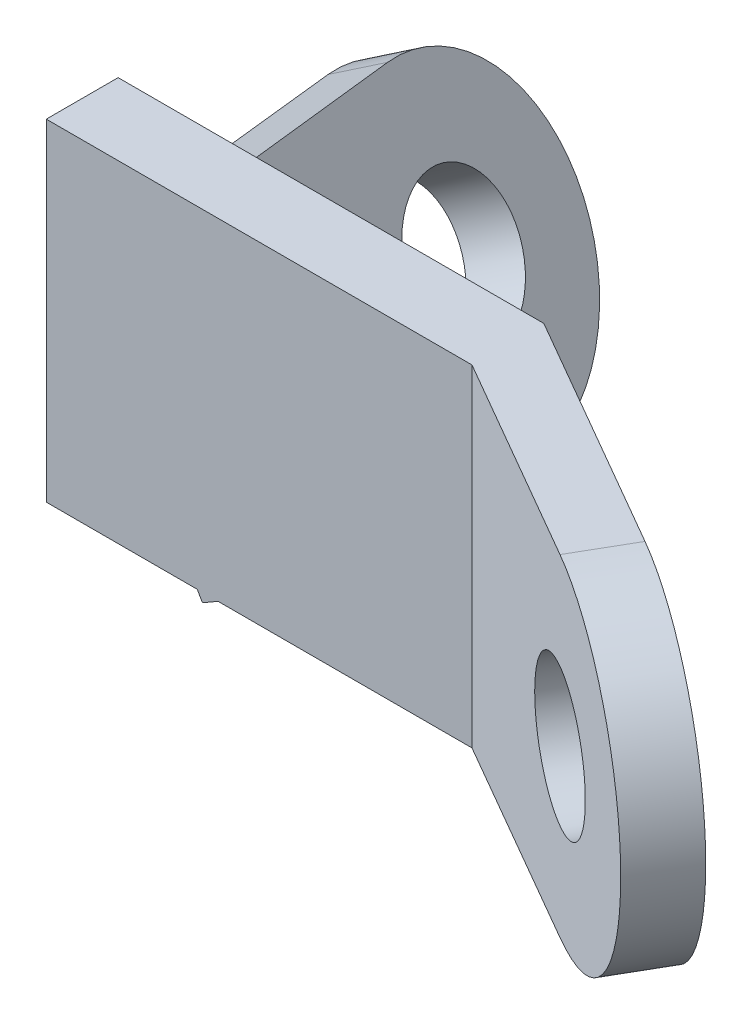
ISO-10303-21;
HEADER;
FILE_DESCRIPTION(('STEP AP214'),'2;1');
FILE_NAME('part.step','',(''),(''),'','','');
FILE_SCHEMA(('AUTOMOTIVE_DESIGN { 1 0 10303 214 1 1 1 1 }'));
ENDSEC;
DATA;
#1=APPLICATION_CONTEXT('core data for automotive mechanical design processes');
#2=APPLICATION_PROTOCOL_DEFINITION('international standard','automotive_design',2000,#1);
#3=PRODUCT_CONTEXT('',#1,'mechanical');
#4=PRODUCT('Part','Part','',(#3));
#5=PRODUCT_RELATED_PRODUCT_CATEGORY('part','',(#4));
#6=PRODUCT_DEFINITION_FORMATION('','',#4);
#7=PRODUCT_DEFINITION_CONTEXT('part definition',#1,'design');
#8=PRODUCT_DEFINITION('design','',#6,#7);
#9=PRODUCT_DEFINITION_SHAPE('','',#8);
#10=(LENGTH_UNIT() NAMED_UNIT(*) SI_UNIT(.MILLI.,.METRE.));
#11=(NAMED_UNIT(*) PLANE_ANGLE_UNIT() SI_UNIT($,.RADIAN.));
#12=(NAMED_UNIT(*) SI_UNIT($,.STERADIAN.) SOLID_ANGLE_UNIT());
#13=UNCERTAINTY_MEASURE_WITH_UNIT(LENGTH_MEASURE(1.E-05),#10,'distance_accuracy_value','');
#14=(GEOMETRIC_REPRESENTATION_CONTEXT(3) GLOBAL_UNCERTAINTY_ASSIGNED_CONTEXT((#13)) GLOBAL_UNIT_ASSIGNED_CONTEXT((#10,
#11,#12)) REPRESENTATION_CONTEXT('',''));
#15=CARTESIAN_POINT('',(0.,0.,0.));
#16=DIRECTION('',(0.,0.,1.));
#17=DIRECTION('',(1.,0.,0.));
#18=AXIS2_PLACEMENT_3D('',#15,#16,#17);
#19=CARTESIAN_POINT('',(-13.5,30.,13.));
#20=DIRECTION('',(0.499999999999998,-0.86602540378444,0.));
#21=DIRECTION('',(0.86602540378444,0.499999999999998,0.));
#22=AXIS2_PLACEMENT_3D('',#19,#20,#21);
#23=PLANE('',#22);
#24=DIRECTION('',(0.836516303737808,0.482962913144532,-0.258819045102525));
#25=VECTOR('',#24,1.);
#26=CARTESIAN_POINT('',(-72.5366146090887,-4.08480533660134,-14.8628456448936));
#27=LINE('',#26,#25);
#28=CARTESIAN_POINT('',(-28.9030249430887,21.1070594027733,-28.3631252703929));
#29=VERTEX_POINT('',#28);
#30=CARTESIAN_POINT('',(-20.6726037773446,25.8588952783596,-30.9096264412501));
#31=VERTEX_POINT('',#30);
#32=EDGE_CURVE('E12',#29,#31,#27,.T.);
#33=ORIENTED_EDGE('',*,*,#32,.F.);
#34=DIRECTION('',(0.219545073021884,0.12675440700844,0.967333076667884));
#35=VECTOR('',#34,1.);
#36=CARTESIAN_POINT('',(-22.0737037228787,25.0499698476439,1.72740792431222));
#37=LINE('',#36,#35);
#38=CARTESIAN_POINT('',(-22.4657547216806,24.8236190979496,0.));
#39=VERTEX_POINT('',#38);
#40=EDGE_CURVE('E74',#29,#39,#37,.T.);
#41=ORIENTED_EDGE('',*,*,#40,.T.);
#42=DIRECTION('',(0.86602540378444,0.499999999999998,0.));
#43=VECTOR('',#42,1.);
#44=CARTESIAN_POINT('',(-16.3653810567665,28.345671475545,0.));
#45=LINE('',#44,#43);
#46=CARTESIAN_POINT('',(-13.5,30.,0.));
#47=VERTEX_POINT('',#46);
#48=EDGE_CURVE('E136',#39,#47,#45,.T.);
#49=ORIENTED_EDGE('',*,*,#48,.T.);
#50=DIRECTION('',(0.224143868042017,0.129409522551262,0.965925826289067));
#51=VECTOR('',#50,1.);
#52=CARTESIAN_POINT('',(-13.691944135042,29.8891810019641,-0.827164262227515));
#53=LINE('',#52,#51);
#54=EDGE_CURVE('E105',#31,#47,#53,.T.);
#55=ORIENTED_EDGE('',*,*,#54,.F.);
#56=EDGE_LOOP('',(#33,#41,#49,#55));
#57=FACE_BOUND('',#56,.T.);
#58=ADVANCED_FACE('F72',(#57),#23,.F.);
#59=CARTESIAN_POINT('',(8.92629627712118,-28.6436051869913,1.72740792431222));
#60=DIRECTION('',(-0.837735018315349,-0.48366653833394,0.253508814016881));
#61=DIRECTION('',(0.499999999999998,-0.86602540378444,0.));
#62=AXIS2_PLACEMENT_3D('',#59,#60,#61);
#63=PLANE('',#62);
#64=CARTESIAN_POINT('',(-15.1530249430887,-2.70863920129879,-28.3631252703929));
#65=DIRECTION('',(-0.837735018315349,-0.48366653833394,0.253508814016881));
#66=DIRECTION('',(-0.219545073021889,-0.126754407008431,-0.967333076667884));
#67=AXIS2_PLACEMENT_3D('',#64,#65,#66);
#68=ELLIPSE('',#67,12.50018862102,12.5);
#69=CARTESIAN_POINT('',(-17.8973797666779,-4.29309319744972,-40.4549711880931));
#70=VERTEX_POINT('',#69);
#71=EDGE_CURVE('E162',#70,#70,#68,.T.);
#72=ORIENTED_EDGE('',*,*,#71,.F.);
#73=EDGE_LOOP('',(#72));
#74=FACE_BOUND('',#73,.T.);
#75=ORIENTED_EDGE('',*,*,#40,.F.);
#76=CARTESIAN_POINT('',(-15.1530249430887,-2.70863920129879,-28.3631252703929));
#77=DIRECTION('',(-0.837735018315349,-0.48366653833394,0.253508814016881));
#78=DIRECTION('',(-0.219545073021889,-0.126754407008431,-0.967333076667884));
#79=AXIS2_PLACEMENT_3D('',#76,#77,#78);
#80=ELLIPSE('',#79,27.500414966244,27.5);
#81=CARTESIAN_POINT('',(-1.40302494308876,-26.5243378053709,-28.3631252703929));
#82=VERTEX_POINT('',#81);
#83=EDGE_CURVE('E86',#29,#82,#80,.T.);
#84=ORIENTED_EDGE('',*,*,#83,.T.);
#85=DIRECTION('',(0.219545073021884,0.12675440700844,0.967333076667884));
#86=VECTOR('',#85,1.);
#87=CARTESIAN_POINT('',(8.37129665810205,-20.8811305977774,14.7033141476249));
#88=LINE('',#87,#86);
#89=CARTESIAN_POINT('',(5.03424527831934,-22.8077781101946,0.));
#90=VERTEX_POINT('',#89);
#91=EDGE_CURVE('E141',#82,#90,#88,.T.);
#92=ORIENTED_EDGE('',*,*,#91,.T.);
#93=DIRECTION('',(-0.499999999999998,0.86602540378444,0.));
#94=VECTOR('',#93,1.);
#95=CARTESIAN_POINT('',(8.53424527831933,-28.8699559366857,0.));
#96=LINE('',#95,#94);
#97=EDGE_CURVE('E139',#90,#39,#96,.T.);
#98=ORIENTED_EDGE('',*,*,#97,.T.);
#99=EDGE_LOOP('',(#75,#84,#92,#98));
#100=FACE_BOUND('',#99,.T.);
#101=ADVANCED_FACE('F143',(#74,#100),#63,.T.);
#102=CARTESIAN_POINT('',(-10.2487113059644,-31.6313972081441,13.));
#103=DIRECTION('',(0.86602540378444,0.499999999999998,0.));
#104=DIRECTION('',(-0.499999999999998,0.86602540378444,0.));
#105=AXIS2_PLACEMENT_3D('',#102,#103,#104);
#106=PLANE('',#105);
#107=DIRECTION('',(-0.499999999999998,0.86602540378444,0.));
#108=VECTOR('',#107,1.);
#109=CARTESIAN_POINT('',(-6.74871130596444,-37.6935750346352,0.));
#110=LINE('',#109,#108);
#111=CARTESIAN_POINT('',(-10.2487113059644,-31.6313972081441,0.));
#112=VERTEX_POINT('',#111);
#113=CARTESIAN_POINT('',(-11.1905989232417,-30.,0.));
#114=VERTEX_POINT('',#113);
#115=EDGE_CURVE('E210',#112,#114,#110,.T.);
#116=ORIENTED_EDGE('',*,*,#115,.F.);
#117=DIRECTION('',(0.,0.,-1.));
#118=VECTOR('',#117,1.);
#119=CARTESIAN_POINT('',(-10.2487113059644,-31.6313972081441,13.));
#120=LINE('',#119,#118);
#121=CARTESIAN_POINT('',(-10.2487113059644,-31.6313972081441,13.));
#122=VERTEX_POINT('',#121);
#123=EDGE_CURVE('E223',#122,#112,#120,.T.);
#124=ORIENTED_EDGE('',*,*,#123,.F.);
#125=DIRECTION('',(0.499999999999998,-0.86602540378444,0.));
#126=VECTOR('',#125,1.);
#127=CARTESIAN_POINT('',(-10.2487113059644,-31.6313972081441,13.));
#128=LINE('',#127,#126);
#129=CARTESIAN_POINT('',(-11.1905989232416,-30.,13.));
#130=VERTEX_POINT('',#129);
#131=EDGE_CURVE('E186',#130,#122,#128,.T.);
#132=ORIENTED_EDGE('',*,*,#131,.F.);
#133=DIRECTION('',(0.,0.,-1.));
#134=VECTOR('',#133,1.);
#135=CARTESIAN_POINT('',(-11.1905989232416,-30.,13.));
#136=LINE('',#135,#134);
#137=EDGE_CURVE('E150',#130,#114,#136,.T.);
#138=ORIENTED_EDGE('',*,*,#137,.T.);
#139=EDGE_LOOP('',(#116,#124,#132,#138));
#140=FACE_BOUND('',#139,.T.);
#141=ADVANCED_FACE('F316',(#140),#106,.F.);
#142=CARTESIAN_POINT('',(13.9999999999999,-17.6313972081442,13.));
#143=DIRECTION('',(-0.499999999999998,0.86602540378444,0.));
#144=DIRECTION('',(-0.86602540378444,-0.499999999999998,0.));
#145=AXIS2_PLACEMENT_3D('',#142,#143,#144);
#146=PLANE('',#145);
#147=ORIENTED_EDGE('',*,*,#91,.F.);
#148=DIRECTION('',(0.836516303737808,0.482962913144532,-0.258819045102525));
#149=VECTOR('',#148,1.);
#150=CARTESIAN_POINT('',(-45.0366146090887,-51.7162025447455,-14.8628456448936));
#151=LINE('',#150,#149);
#152=CARTESIAN_POINT('',(6.82739622265535,-21.7725019297846,-30.9096264412502));
#153=VERTEX_POINT('',#152);
#154=EDGE_CURVE('E235',#82,#153,#151,.T.);
#155=ORIENTED_EDGE('',*,*,#154,.T.);
#156=DIRECTION('',(0.224143868042017,0.129409522551262,0.965925826289067));
#157=VECTOR('',#156,1.);
#158=CARTESIAN_POINT('',(16.8145825622994,-16.0063972081442,12.1291651245988));
#159=LINE('',#158,#157);
#160=CARTESIAN_POINT('',(13.9999999999999,-17.6313972081442,0.));
#161=VERTEX_POINT('',#160);
#162=EDGE_CURVE('E157',#153,#161,#159,.T.);
#163=ORIENTED_EDGE('',*,*,#162,.T.);
#164=DIRECTION('',(-0.86602540378444,-0.499999999999998,0.));
#165=VECTOR('',#164,1.);
#166=CARTESIAN_POINT('',(11.1346189432334,-19.2857257325992,0.));
#167=LINE('',#166,#165);
#168=EDGE_CURVE('E163',#161,#90,#167,.T.);
#169=ORIENTED_EDGE('',*,*,#168,.T.);
#170=EDGE_LOOP('',(#147,#155,#163,#169));
#171=FACE_BOUND('',#170,.T.);
#172=ADVANCED_FACE('F261',(#171),#146,.F.);
#173=CARTESIAN_POINT('',(-38.5,-30.,13.));
#174=DIRECTION('',(0.,1.,0.));
#175=DIRECTION('',(0.,0.,1.));
#176=AXIS2_PLACEMENT_3D('',#173,#174,#175);
#177=PLANE('',#176);
#178=ORIENTED_EDGE('',*,*,#137,.F.);
#179=DIRECTION('',(1.,0.,0.));
#180=VECTOR('',#179,1.);
#181=CARTESIAN_POINT('',(-38.5,-30.,13.));
#182=LINE('',#181,#180);
#183=CARTESIAN_POINT('',(-38.5,-30.,13.));
#184=VERTEX_POINT('',#183);
#185=EDGE_CURVE('E190',#184,#130,#182,.T.);
#186=ORIENTED_EDGE('',*,*,#185,.F.);
#187=DIRECTION('',(0.,0.,-1.));
#188=VECTOR('',#187,1.);
#189=CARTESIAN_POINT('',(-38.5,-30.,13.));
#190=LINE('',#189,#188);
#191=CARTESIAN_POINT('',(-38.5,-30.,0.));
#192=VERTEX_POINT('',#191);
#193=EDGE_CURVE('E167',#184,#192,#190,.T.);
#194=ORIENTED_EDGE('',*,*,#193,.T.);
#195=DIRECTION('',(1.,0.,0.));
#196=VECTOR('',#195,1.);
#197=CARTESIAN_POINT('',(-38.5,-30.,0.));
#198=LINE('',#197,#196);
#199=EDGE_CURVE('E174',#192,#114,#198,.T.);
#200=ORIENTED_EDGE('',*,*,#199,.T.);
#201=EDGE_LOOP('',(#178,#186,#194,#200));
#202=FACE_BOUND('',#201,.T.);
#203=ADVANCED_FACE('F315',(#202),#177,.F.);
#204=DIRECTION('',(0.,0.,1.));
#205=VECTOR('',#204,1.);
#206=CARTESIAN_POINT('',(-7.42304845413277,-30.,13.));
#207=LINE('',#206,#205);
#208=CARTESIAN_POINT('',(-7.42304845413277,-30.,0.));
#209=VERTEX_POINT('',#208);
#210=CARTESIAN_POINT('',(-7.42304845413277,-30.,13.));
#211=VERTEX_POINT('',#210);
#212=EDGE_CURVE('E233',#209,#211,#207,.T.);
#213=ORIENTED_EDGE('',*,*,#212,.F.);
#214=CARTESIAN_POINT('',(38.5,-30.,0.));
#215=VERTEX_POINT('',#214);
#216=EDGE_CURVE('E180',#209,#215,#198,.T.);
#217=ORIENTED_EDGE('',*,*,#216,.T.);
#218=DIRECTION('',(0.866025403784442,0.,0.499999999999994));
#219=VECTOR('',#218,1.);
#220=CARTESIAN_POINT('',(9.62499999999978,-30.,-16.6709890228503));
#221=LINE('',#220,#219);
#222=CARTESIAN_POINT('',(81.8012701892221,-30.,24.9999999999997));
#223=VERTEX_POINT('',#222);
#224=EDGE_CURVE('E203',#215,#223,#221,.T.);
#225=ORIENTED_EDGE('',*,*,#224,.T.);
#226=DIRECTION('',(0.499999999999994,0.,-0.866025403784442));
#227=VECTOR('',#226,1.);
#228=CARTESIAN_POINT('',(75.3012701892222,-30.,36.2583302491974));
#229=LINE('',#228,#227);
#230=CARTESIAN_POINT('',(76.1721050646233,-30.,34.7499999999998));
#231=VERTEX_POINT('',#230);
#232=EDGE_CURVE('E225',#231,#223,#229,.T.);
#233=ORIENTED_EDGE('',*,*,#232,.F.);
#234=DIRECTION('',(-0.866025403784442,0.,-0.499999999999994));
#235=VECTOR('',#234,1.);
#236=CARTESIAN_POINT('',(3.99583487540097,-30.,-6.92098902285024));
#237=LINE('',#236,#235);
#238=CARTESIAN_POINT('',(38.5,-30.,13.));
#239=VERTEX_POINT('',#238);
#240=EDGE_CURVE('E204',#231,#239,#237,.T.);
#241=ORIENTED_EDGE('',*,*,#240,.T.);
#242=EDGE_CURVE('E195',#211,#239,#182,.T.);
#243=ORIENTED_EDGE('',*,*,#242,.F.);
#244=EDGE_LOOP('',(#213,#217,#225,#233,#241,#243));
#245=FACE_BOUND('',#244,.T.);
#246=ADVANCED_FACE('F330',(#245),#177,.F.);
#247=CARTESIAN_POINT('',(0.,0.,0.));
#248=DIRECTION('',(0.,0.,1.));
#249=DIRECTION('',(1.,0.,0.));
#250=AXIS2_PLACEMENT_3D('',#247,#248,#249);
#251=PLANE('',#250);
#252=ORIENTED_EDGE('',*,*,#48,.F.);
#253=ORIENTED_EDGE('',*,*,#97,.F.);
#254=ORIENTED_EDGE('',*,*,#168,.F.);
#255=DIRECTION('',(0.499999999999998,-0.86602540378444,0.));
#256=VECTOR('',#255,1.);
#257=CARTESIAN_POINT('',(2.86538105676651,1.65432852445499,0.));
#258=LINE('',#257,#256);
#259=EDGE_CURVE('E161',#47,#161,#258,.T.);
#260=ORIENTED_EDGE('',*,*,#259,.F.);
#261=DIRECTION('',(-1.,0.,0.));
#262=VECTOR('',#261,1.);
#263=CARTESIAN_POINT('',(-38.5,30.,0.));
#264=LINE('',#263,#262);
#265=CARTESIAN_POINT('',(38.5,30.,0.));
#266=VERTEX_POINT('',#265);
#267=EDGE_CURVE('E182',#266,#47,#264,.T.);
#268=ORIENTED_EDGE('',*,*,#267,.F.);
#269=DIRECTION('',(0.,1.,0.));
#270=VECTOR('',#269,1.);
#271=CARTESIAN_POINT('',(38.5,30.,0.));
#272=LINE('',#271,#270);
#273=EDGE_CURVE('E181',#215,#266,#272,.T.);
#274=ORIENTED_EDGE('',*,*,#273,.F.);
#275=ORIENTED_EDGE('',*,*,#216,.F.);
#276=DIRECTION('',(0.86602540378444,0.499999999999998,0.));
#277=VECTOR('',#276,1.);
#278=CARTESIAN_POINT('',(13.9999999999999,-17.6313972081442,0.));
#279=LINE('',#278,#277);
#280=EDGE_CURVE('E112',#112,#209,#279,.T.);
#281=ORIENTED_EDGE('',*,*,#280,.F.);
#282=ORIENTED_EDGE('',*,*,#115,.T.);
#283=ORIENTED_EDGE('',*,*,#199,.F.);
#284=DIRECTION('',(0.,-1.,0.));
#285=VECTOR('',#284,1.);
#286=CARTESIAN_POINT('',(-38.5,30.,0.));
#287=LINE('',#286,#285);
#288=CARTESIAN_POINT('',(-38.5,30.,0.));
#289=VERTEX_POINT('',#288);
#290=EDGE_CURVE('E172',#289,#192,#287,.T.);
#291=ORIENTED_EDGE('',*,*,#290,.F.);
#292=EDGE_CURVE('E153',#47,#289,#264,.T.);
#293=ORIENTED_EDGE('',*,*,#292,.F.);
#294=EDGE_LOOP('',(#252,#253,#254,#260,#268,#274,#275,#281,#282,#283,#291,#293));
#295=FACE_BOUND('',#294,.T.);
#296=ADVANCED_FACE('F147',(#295),#251,.F.);
#297=CARTESIAN_POINT('',(3.99583487540097,30.,-6.92098902285024));
#298=DIRECTION('',(-0.499999999999994,0.,0.866025403784442));
#299=DIRECTION('',(0.866025403784442,0.,0.499999999999994));
#300=AXIS2_PLACEMENT_3D('',#297,#298,#299);
#301=PLANE('',#300);
#302=CARTESIAN_POINT('',(76.1721050646233,0.,34.7499999999998));
#303=DIRECTION('',(-0.499999999999994,0.,0.866025403784442));
#304=DIRECTION('',(0.866025403784442,0.,0.499999999999994));
#305=AXIS2_PLACEMENT_3D('',#302,#303,#304);
#306=CIRCLE('',#305,12.5);
#307=CARTESIAN_POINT('',(65.3467875173178,0.,28.4999999999999));
#308=VERTEX_POINT('',#307);
#309=EDGE_CURVE('E199',#308,#308,#306,.T.);
#310=ORIENTED_EDGE('',*,*,#309,.F.);
#311=EDGE_LOOP('',(#310));
#312=FACE_BOUND('',#311,.T.);
#313=ORIENTED_EDGE('',*,*,#240,.F.);
#314=CARTESIAN_POINT('',(76.1721050646233,0.,34.7499999999998));
#315=DIRECTION('',(-0.499999999999994,0.,0.866025403784442));
#316=DIRECTION('',(0.866025403784442,0.,0.499999999999994));
#317=AXIS2_PLACEMENT_3D('',#314,#315,#316);
#318=CIRCLE('',#317,30.);
#319=CARTESIAN_POINT('',(76.1721050646233,30.,34.7499999999998));
#320=VERTEX_POINT('',#319);
#321=EDGE_CURVE('E212',#231,#320,#318,.T.);
#322=ORIENTED_EDGE('',*,*,#321,.T.);
#323=DIRECTION('',(-0.866025403784442,0.,-0.499999999999994));
#324=VECTOR('',#323,1.);
#325=CARTESIAN_POINT('',(3.99583487540097,30.,-6.92098902285024));
#326=LINE('',#325,#324);
#327=CARTESIAN_POINT('',(38.5,30.,13.));
#328=VERTEX_POINT('',#327);
#329=EDGE_CURVE('E211',#320,#328,#326,.T.);
#330=ORIENTED_EDGE('',*,*,#329,.T.);
#331=DIRECTION('',(0.,1.,0.));
#332=VECTOR('',#331,1.);
#333=CARTESIAN_POINT('',(38.5,30.,13.));
#334=LINE('',#333,#332);
#335=EDGE_CURVE('E197',#239,#328,#334,.T.);
#336=ORIENTED_EDGE('',*,*,#335,.F.);
#337=EDGE_LOOP('',(#313,#322,#330,#336));
#338=FACE_BOUND('',#337,.T.);
#339=ADVANCED_FACE('F324',(#312,#338),#301,.T.);
#340=CARTESIAN_POINT('',(9.62499999999978,30.,-16.6709890228503));
#341=DIRECTION('',(0.499999999999994,0.,-0.866025403784442));
#342=DIRECTION('',(-0.866025403784442,0.,-0.499999999999994));
#343=AXIS2_PLACEMENT_3D('',#340,#341,#342);
#344=PLANE('',#343);
#345=CARTESIAN_POINT('',(81.8012701892221,0.,24.9999999999997));
#346=DIRECTION('',(0.499999999999994,0.,-0.866025403784442));
#347=DIRECTION('',(-0.866025403784442,0.,-0.499999999999994));
#348=AXIS2_PLACEMENT_3D('',#345,#346,#347);
#349=CIRCLE('',#348,12.5);
#350=CARTESIAN_POINT('',(70.9759526419166,0.,18.7499999999998));
#351=VERTEX_POINT('',#350);
#352=EDGE_CURVE('E220',#351,#351,#349,.T.);
#353=ORIENTED_EDGE('',*,*,#352,.F.);
#354=EDGE_LOOP('',(#353));
#355=FACE_BOUND('',#354,.T.);
#356=DIRECTION('',(0.866025403784442,0.,0.499999999999994));
#357=VECTOR('',#356,1.);
#358=CARTESIAN_POINT('',(9.62499999999978,30.,-16.6709890228503));
#359=LINE('',#358,#357);
#360=CARTESIAN_POINT('',(81.8012701892221,30.,24.9999999999997));
#361=VERTEX_POINT('',#360);
#362=EDGE_CURVE('E208',#266,#361,#359,.T.);
#363=ORIENTED_EDGE('',*,*,#362,.T.);
#364=CARTESIAN_POINT('',(81.8012701892221,0.,24.9999999999997));
#365=DIRECTION('',(0.499999999999994,0.,-0.866025403784442));
#366=DIRECTION('',(-0.866025403784442,0.,-0.499999999999994));
#367=AXIS2_PLACEMENT_3D('',#364,#365,#366);
#368=CIRCLE('',#367,30.);
#369=EDGE_CURVE('E187',#361,#223,#368,.T.);
#370=ORIENTED_EDGE('',*,*,#369,.T.);
#371=ORIENTED_EDGE('',*,*,#224,.F.);
#372=ORIENTED_EDGE('',*,*,#273,.T.);
#373=EDGE_LOOP('',(#363,#370,#371,#372));
#374=FACE_BOUND('',#373,.T.);
#375=ADVANCED_FACE('F301',(#355,#374),#344,.T.);
#376=CARTESIAN_POINT('',(-38.5,30.,13.));
#377=DIRECTION('',(0.,-1.,0.));
#378=DIRECTION('',(0.,0.,-1.));
#379=AXIS2_PLACEMENT_3D('',#376,#377,#378);
#380=PLANE('',#379);
#381=ORIENTED_EDGE('',*,*,#267,.T.);
#382=ORIENTED_EDGE('',*,*,#292,.T.);
#383=DIRECTION('',(0.,0.,-1.));
#384=VECTOR('',#383,1.);
#385=CARTESIAN_POINT('',(-38.5,30.,13.));
#386=LINE('',#385,#384);
#387=CARTESIAN_POINT('',(-38.5,30.,13.));
#388=VERTEX_POINT('',#387);
#389=EDGE_CURVE('E170',#388,#289,#386,.T.);
#390=ORIENTED_EDGE('',*,*,#389,.F.);
#391=DIRECTION('',(-1.,0.,0.));
#392=VECTOR('',#391,1.);
#393=CARTESIAN_POINT('',(-38.5,30.,13.));
#394=LINE('',#393,#392);
#395=EDGE_CURVE('E168',#328,#388,#394,.T.);
#396=ORIENTED_EDGE('',*,*,#395,.F.);
#397=ORIENTED_EDGE('',*,*,#329,.F.);
#398=DIRECTION('',(0.499999999999994,0.,-0.866025403784442));
#399=VECTOR('',#398,1.);
#400=CARTESIAN_POINT('',(75.3012701892222,30.,36.2583302491974));
#401=LINE('',#400,#399);
#402=EDGE_CURVE('E179',#320,#361,#401,.T.);
#403=ORIENTED_EDGE('',*,*,#402,.T.);
#404=ORIENTED_EDGE('',*,*,#362,.F.);
#405=EDGE_LOOP('',(#381,#382,#390,#396,#397,#403,#404));
#406=FACE_BOUND('',#405,.T.);
#407=ADVANCED_FACE('F299',(#406),#380,.F.);
#408=CARTESIAN_POINT('',(-38.5,30.,13.));
#409=DIRECTION('',(1.,0.,0.));
#410=DIRECTION('',(0.,1.,0.));
#411=AXIS2_PLACEMENT_3D('',#408,#409,#410);
#412=PLANE('',#411);
#413=ORIENTED_EDGE('',*,*,#290,.T.);
#414=ORIENTED_EDGE('',*,*,#193,.F.);
#415=DIRECTION('',(0.,-1.,0.));
#416=VECTOR('',#415,1.);
#417=CARTESIAN_POINT('',(-38.5,30.,13.));
#418=LINE('',#417,#416);
#419=EDGE_CURVE('E191',#388,#184,#418,.T.);
#420=ORIENTED_EDGE('',*,*,#419,.F.);
#421=ORIENTED_EDGE('',*,*,#389,.T.);
#422=EDGE_LOOP('',(#413,#414,#420,#421));
#423=FACE_BOUND('',#422,.T.);
#424=ADVANCED_FACE('F307',(#423),#412,.F.);
#425=CARTESIAN_POINT('',(0.,0.,13.));
#426=DIRECTION('',(0.,0.,1.));
#427=DIRECTION('',(1.,0.,0.));
#428=AXIS2_PLACEMENT_3D('',#425,#426,#427);
#429=PLANE('',#428);
#430=ORIENTED_EDGE('',*,*,#395,.T.);
#431=ORIENTED_EDGE('',*,*,#419,.T.);
#432=ORIENTED_EDGE('',*,*,#185,.T.);
#433=ORIENTED_EDGE('',*,*,#131,.T.);
#434=DIRECTION('',(0.86602540378444,0.499999999999998,0.));
#435=VECTOR('',#434,1.);
#436=CARTESIAN_POINT('',(13.9999999999999,-17.6313972081442,13.));
#437=LINE('',#436,#435);
#438=EDGE_CURVE('E240',#122,#211,#437,.T.);
#439=ORIENTED_EDGE('',*,*,#438,.T.);
#440=ORIENTED_EDGE('',*,*,#242,.T.);
#441=ORIENTED_EDGE('',*,*,#335,.T.);
#442=EDGE_LOOP('',(#430,#431,#432,#433,#439,#440,#441));
#443=FACE_BOUND('',#442,.T.);
#444=ADVANCED_FACE('F319',(#443),#429,.T.);
#445=CARTESIAN_POINT('',(75.3012701892222,0.,36.2583302491974));
#446=DIRECTION('',(0.499999999999994,0.,-0.866025403784442));
#447=DIRECTION('',(-0.866025403784442,0.,-0.499999999999994));
#448=AXIS2_PLACEMENT_3D('',#445,#446,#447);
#449=CYLINDRICAL_SURFACE('',#448,12.5);
#450=CARTESIAN_POINT('',(65.3467875173178,0.,28.4999999999999));
#451=CARTESIAN_POINT('',(65.4054246540323,0.,28.3984374999999));
#452=CARTESIAN_POINT('',(65.4640617907469,0.,28.2968749999999));
#453=CARTESIAN_POINT('',(65.581336064176,0.,28.0937499999999));
#454=CARTESIAN_POINT('',(65.6399732008906,0.,27.9921874999999));
#455=CARTESIAN_POINT('',(65.7572474743198,0.,27.7890624999999));
#456=CARTESIAN_POINT('',(65.8158846110343,0.,27.6874999999999));
#457=CARTESIAN_POINT('',(65.9331588844635,0.,27.4843749999999));
#458=CARTESIAN_POINT('',(65.991796021178,0.,27.3828124999999));
#459=CARTESIAN_POINT('',(66.1090702946072,0.,27.1796874999998));
#460=CARTESIAN_POINT('',(66.1677074313217,0.,27.0781249999998));
#461=CARTESIAN_POINT('',(66.2849817047509,0.,26.8749999999998));
#462=CARTESIAN_POINT('',(66.3436188414655,0.,26.7734374999998));
#463=CARTESIAN_POINT('',(66.4608931148946,0.,26.5703124999998));
#464=CARTESIAN_POINT('',(66.5195302516092,0.,26.4687499999998));
#465=CARTESIAN_POINT('',(66.6368045250383,0.,26.2656249999998));
#466=CARTESIAN_POINT('',(66.6954416617529,0.,26.1640624999998));
#467=CARTESIAN_POINT('',(66.812715935182,0.,25.9609374999998));
#468=CARTESIAN_POINT('',(66.8713530718966,0.,25.8593749999998));
#469=CARTESIAN_POINT('',(66.9886273453258,0.,25.6562499999998));
#470=CARTESIAN_POINT('',(67.0472644820403,0.,25.5546874999998));
#471=CARTESIAN_POINT('',(67.1645387554695,0.,25.3515624999998));
#472=CARTESIAN_POINT('',(67.223175892184,0.,25.2499999999998));
#473=CARTESIAN_POINT('',(67.3404501656132,0.,25.0468749999998));
#474=CARTESIAN_POINT('',(67.3990873023277,0.,24.9453124999998));
#475=CARTESIAN_POINT('',(67.5163615757569,0.,24.7421874999998));
#476=CARTESIAN_POINT('',(67.5749987124715,0.,24.6406249999998));
#477=CARTESIAN_POINT('',(67.6922729859006,0.,24.4374999999998));
#478=CARTESIAN_POINT('',(67.7509101226152,0.,24.3359374999998));
#479=CARTESIAN_POINT('',(67.8681843960443,0.,24.1328124999998));
#480=CARTESIAN_POINT('',(67.9268215327589,0.,24.0312499999998));
#481=CARTESIAN_POINT('',(68.044095806188,0.,23.8281249999998));
#482=CARTESIAN_POINT('',(68.1027329429026,0.,23.7265624999998));
#483=CARTESIAN_POINT('',(68.2200072163317,0.,23.5234374999998));
#484=CARTESIAN_POINT('',(68.2786443530463,0.,23.4218749999998));
#485=CARTESIAN_POINT('',(68.3959186264754,0.,23.2187499999998));
#486=CARTESIAN_POINT('',(68.45455576319,0.,23.1171874999998));
#487=CARTESIAN_POINT('',(68.5718300366192,0.,22.9140624999998));
#488=CARTESIAN_POINT('',(68.6304671733337,0.,22.8124999999998));
#489=CARTESIAN_POINT('',(68.7477414467629,0.,22.6093749999998));
#490=CARTESIAN_POINT('',(68.8063785834775,0.,22.5078124999998));
#491=CARTESIAN_POINT('',(68.9236528569066,0.,22.3046874999998));
#492=CARTESIAN_POINT('',(68.9822899936212,0.,22.2031249999998));
#493=CARTESIAN_POINT('',(69.0995642670503,0.,21.9999999999998));
#494=CARTESIAN_POINT('',(69.1582014037649,0.,21.8984374999998));
#495=CARTESIAN_POINT('',(69.275475677194,0.,21.6953124999998));
#496=CARTESIAN_POINT('',(69.3341128139086,0.,21.5937499999998));
#497=CARTESIAN_POINT('',(69.4513870873377,0.,21.3906249999998));
#498=CARTESIAN_POINT('',(69.5100242240523,0.,21.2890624999998));
#499=CARTESIAN_POINT('',(69.6272984974814,0.,21.0859374999998));
#500=CARTESIAN_POINT('',(69.685935634196,0.,20.9843749999998));
#501=CARTESIAN_POINT('',(69.8032099076252,0.,20.7812499999998));
#502=CARTESIAN_POINT('',(69.8618470443397,0.,20.6796874999998));
#503=CARTESIAN_POINT('',(69.9791213177689,0.,20.4765624999998));
#504=CARTESIAN_POINT('',(70.0377584544834,0.,20.3749999999998));
#505=CARTESIAN_POINT('',(70.1550327279126,0.,20.1718749999998));
#506=CARTESIAN_POINT('',(70.2136698646271,0.,20.0703124999998));
#507=CARTESIAN_POINT('',(70.3309441380563,0.,19.8671874999998));
#508=CARTESIAN_POINT('',(70.3895812747709,0.,19.7656249999998));
#509=CARTESIAN_POINT('',(70.5068555482,0.,19.5624999999998));
#510=CARTESIAN_POINT('',(70.5654926849146,0.,19.4609374999998));
#511=CARTESIAN_POINT('',(70.6827669583437,0.,19.2578124999998));
#512=CARTESIAN_POINT('',(70.7414040950583,0.,19.1562499999998));
#513=CARTESIAN_POINT('',(70.8586783684874,0.,18.9531249999998));
#514=CARTESIAN_POINT('',(70.917315505202,0.,18.8515624999998));
#515=CARTESIAN_POINT('',(70.9759526419166,0.,18.7499999999998));
#516=B_SPLINE_CURVE_WITH_KNOTS('',3,(#450,#451,#452,#453,#454,#455,#456,#457,#458,#459,#460,
#461,#462,#463,#464,#465,#466,#467,#468,#469,#470,#471,#472,#473,#474,#475,#476,#477,#478,#479,
#480,#481,#482,#483,#484,#485,#486,#487,#488,#489,#490,#491,#492,#493,#494,#495,#496,#497,#498,
#499,#500,#501,#502,#503,#504,#505,#506,#507,#508,#509,#510,#511,#512,#513,#514,#515),
.UNSPECIFIED.,.F.,.F.,(4,2,2,2,2,2,2,2,2,2,2,2,2,2,2,2,2,2,2,2,2,2,2,2,2,2,2,2,2,2,2,2,4),(0.,
0.351822820287431,0.703645640574859,1.05546846086229,1.40729128114972,1.75911410143715,
2.11093692172458,2.46275974201201,2.81458256229944,3.16640538258687,3.5182282028743,
3.87005102316173,4.22187384344916,4.57369666373659,4.92551948402402,5.27734230431145,
5.62916512459888,5.98098794488631,6.33281076517374,6.68463358546117,7.0364564057486,
7.38827922603603,7.74010204632346,8.09192486661088,8.44374768689832,8.79557050718576,
9.14739332747318,9.49921614776061,9.85103896804804,10.2028617883355,10.5546846086229,
10.9065074289103,11.2583302491978),.UNSPECIFIED.);
#517=EDGE_CURVE('BSEAM335',#308,#351,#516,.T.);
#518=ORIENTED_EDGE('',*,*,#309,.T.);
#519=ORIENTED_EDGE('',*,*,#352,.T.);
#520=ORIENTED_EDGE('',*,*,#517,.T.);
#521=ORIENTED_EDGE('',*,*,#517,.F.);
#522=EDGE_LOOP('',(#518,#520,#519,#521));
#523=FACE_BOUND('',#522,.T.);
#524=ADVANCED_FACE('F335',(#523),#449,.F.);
#525=CARTESIAN_POINT('',(75.3012701892222,0.,36.2583302491974));
#526=DIRECTION('',(0.499999999999994,0.,-0.866025403784442));
#527=DIRECTION('',(-0.866025403784442,0.,-0.499999999999994));
#528=AXIS2_PLACEMENT_3D('',#525,#526,#527);
#529=CYLINDRICAL_SURFACE('',#528,30.);
#530=ORIENTED_EDGE('',*,*,#232,.T.);
#531=ORIENTED_EDGE('',*,*,#369,.F.);
#532=ORIENTED_EDGE('',*,*,#402,.F.);
#533=ORIENTED_EDGE('',*,*,#321,.F.);
#534=EDGE_LOOP('',(#530,#531,#532,#533));
#535=FACE_BOUND('',#534,.T.);
#536=ADVANCED_FACE('F295',(#535),#529,.T.);
#537=ORIENTED_EDGE('',*,*,#123,.T.);
#538=ORIENTED_EDGE('',*,*,#280,.T.);
#539=ORIENTED_EDGE('',*,*,#212,.T.);
#540=ORIENTED_EDGE('',*,*,#438,.F.);
#541=EDGE_LOOP('',(#537,#538,#539,#540));
#542=FACE_BOUND('',#541,.T.);
#543=ADVANCED_FACE('F258',(#542),#146,.F.);
#544=CARTESIAN_POINT('',(17.3080558649579,-23.8043940326711,-0.827164262227515));
#545=DIRECTION('',(-0.836516303737808,-0.482962913144532,0.258819045102525));
#546=DIRECTION('',(0.499999999999998,-0.86602540378444,0.));
#547=AXIS2_PLACEMENT_3D('',#544,#545,#546);
#548=PLANE('',#547);
#549=CARTESIAN_POINT('',(-6.92260377734461,2.04319667428754,-30.9096264412502));
#550=DIRECTION('',(0.836516303737808,0.482962913144532,-0.258819045102525));
#551=DIRECTION('',(-0.499999999999998,0.86602540378444,0.));
#552=AXIS2_PLACEMENT_3D('',#549,#550,#551);
#553=CIRCLE('',#552,12.5);
#554=CARTESIAN_POINT('',(-13.1726037773446,12.868514221593,-30.9096264412502));
#555=VERTEX_POINT('',#554);
#556=EDGE_CURVE('E76',#555,#555,#553,.T.);
#557=ORIENTED_EDGE('',*,*,#556,.F.);
#558=EDGE_LOOP('',(#557));
#559=FACE_BOUND('',#558,.T.);
#560=ORIENTED_EDGE('',*,*,#162,.F.);
#561=CARTESIAN_POINT('',(-6.92260377734461,2.04319667428754,-30.9096264412502));
#562=DIRECTION('',(0.836516303737808,0.482962913144532,-0.258819045102525));
#563=DIRECTION('',(-0.499999999999998,0.86602540378444,0.));
#564=AXIS2_PLACEMENT_3D('',#561,#562,#563);
#565=CIRCLE('',#564,27.5);
#566=EDGE_CURVE('E234',#153,#31,#565,.T.);
#567=ORIENTED_EDGE('',*,*,#566,.T.);
#568=ORIENTED_EDGE('',*,*,#54,.T.);
#569=ORIENTED_EDGE('',*,*,#259,.T.);
#570=EDGE_LOOP('',(#560,#567,#568,#569));
#571=FACE_BOUND('',#570,.T.);
#572=ADVANCED_FACE('F255',(#559,#571),#548,.F.);
#573=CARTESIAN_POINT('',(-58.7866146090887,-27.9005039406734,-14.8628456448936));
#574=DIRECTION('',(0.836516303737808,0.482962913144532,-0.258819045102525));
#575=DIRECTION('',(-0.499999999999998,0.86602540378444,0.));
#576=AXIS2_PLACEMENT_3D('',#573,#574,#575);
#577=CYLINDRICAL_SURFACE('',#576,12.5);
#578=ORIENTED_EDGE('',*,*,#71,.T.);
#579=EDGE_LOOP('',(#578));
#580=FACE_BOUND('',#579,.T.);
#581=ORIENTED_EDGE('',*,*,#556,.T.);
#582=EDGE_LOOP('',(#581));
#583=FACE_BOUND('',#582,.T.);
#584=ADVANCED_FACE('F252',(#580,#583),#577,.F.);
#585=CARTESIAN_POINT('',(-58.7866146090887,-27.9005039406734,-14.8628456448936));
#586=DIRECTION('',(0.836516303737808,0.482962913144532,-0.258819045102525));
#587=DIRECTION('',(-0.499999999999998,0.86602540378444,0.));
#588=AXIS2_PLACEMENT_3D('',#585,#586,#587);
#589=CYLINDRICAL_SURFACE('',#588,27.5);
#590=ORIENTED_EDGE('',*,*,#32,.T.);
#591=ORIENTED_EDGE('',*,*,#566,.F.);
#592=ORIENTED_EDGE('',*,*,#154,.F.);
#593=ORIENTED_EDGE('',*,*,#83,.F.);
#594=EDGE_LOOP('',(#590,#591,#592,#593));
#595=FACE_BOUND('',#594,.T.);
#596=ADVANCED_FACE('F349',(#595),#589,.T.);
#597=CLOSED_SHELL('',(#58,#101,#141,#172,#203,#246,#296,#339,#375,#407,#424,#444,#524,#536,#543,
#572,#584,#596));
#598=MANIFOLD_SOLID_BREP('B2',#597);
#599=ADVANCED_BREP_SHAPE_REPRESENTATION('',(#18,#598),#14);
#600=SHAPE_DEFINITION_REPRESENTATION(#9,#599);
ENDSEC;
END-ISO-10303-21;
